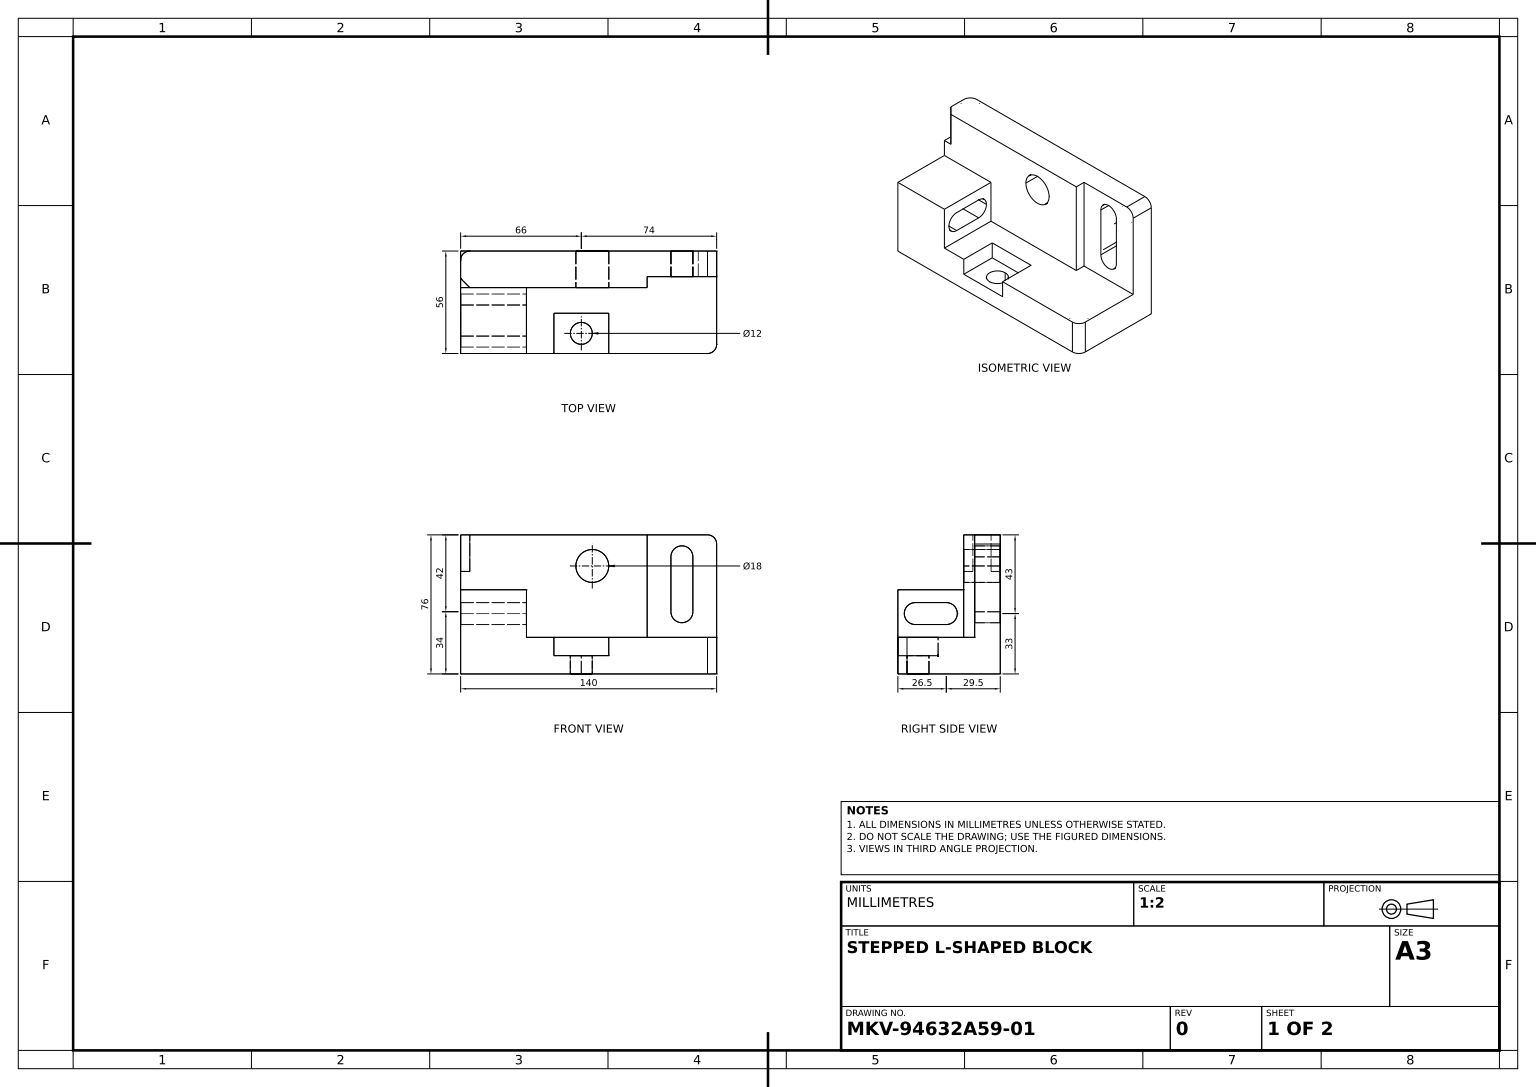
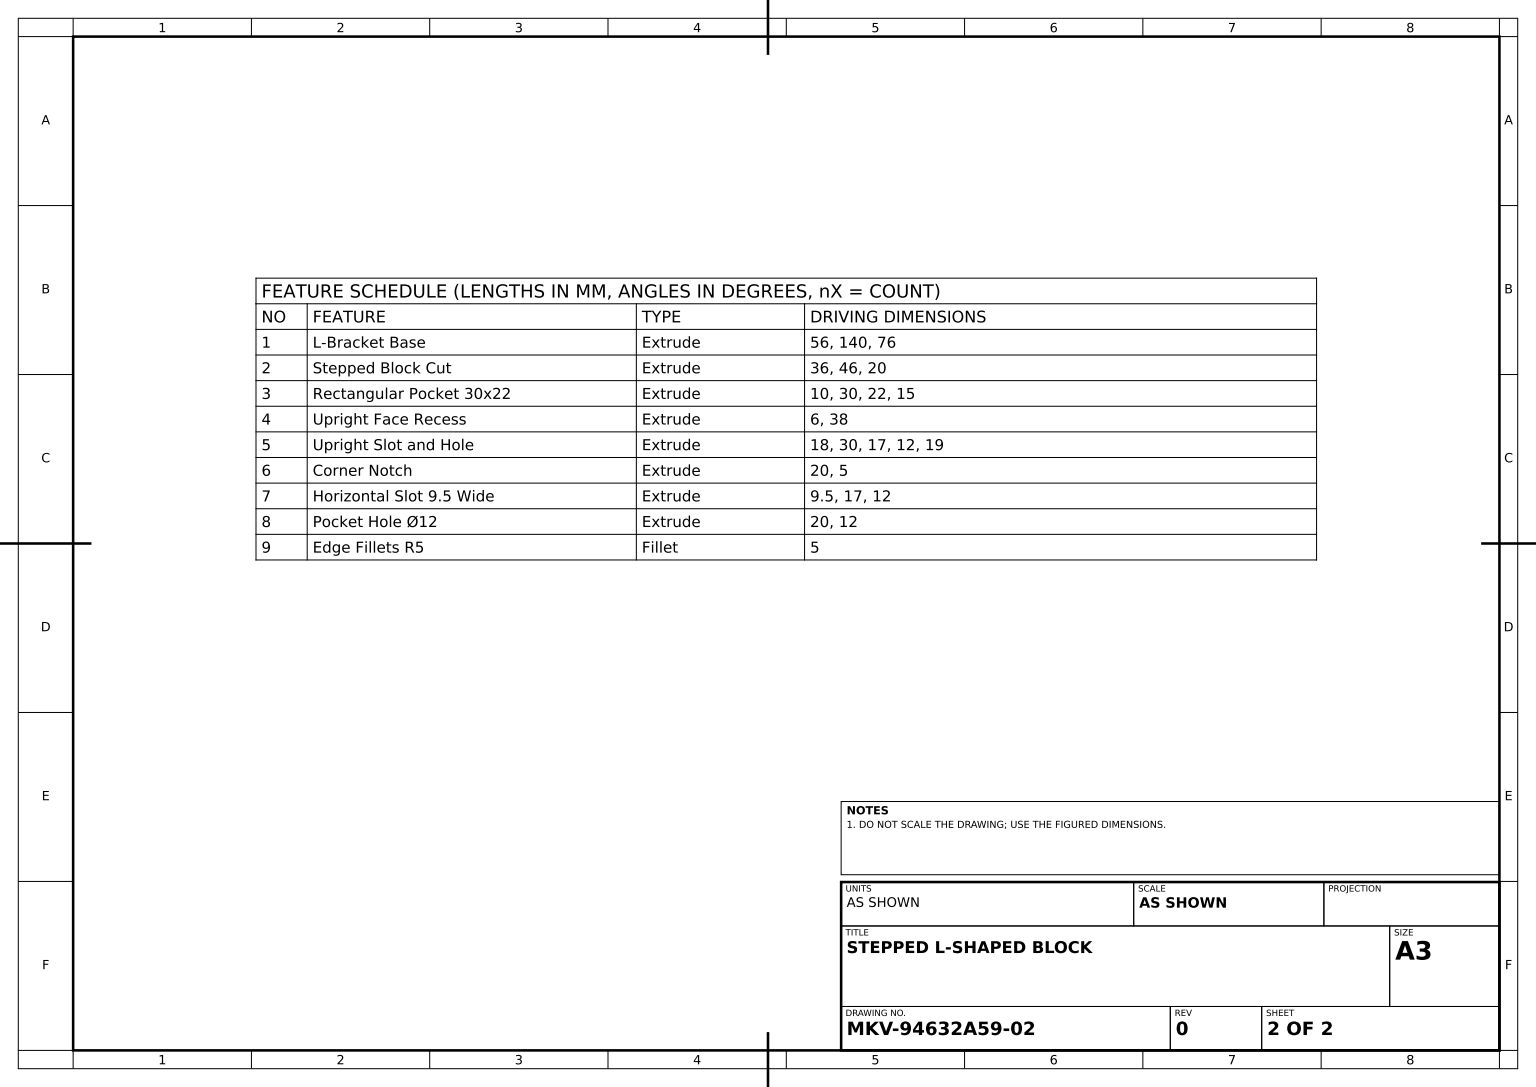
from build123d import *

# Parameters (mm, degrees)
L_BRACKET_PROFILE_SKETCH_W     = 140
L_BRACKET_PROFILE_SKETCH_H     = 76
L_BRACKET_BASE_DEPTH           = 28
STEPPED_BLOCK_CUT_DEPTH        = 36
RECTANGULAR_POCKET_SKETCH_W    = 30
RECTANGULAR_POCKET_SKETCH_H    = 22
RECTANGULAR_POCKET_30X22_DEPTH = 10
UPRIGHT_RECESS_SKETCH_W        = 38
UPRIGHT_RECESS_SKETCH_H        = 56
UPRIGHT_FACE_RECESS_DEPTH      = 6
UPRIGHT_SLOT_AND_HOLE_SKETCH_R = 9
UPRIGHT_SLOT_AND_HOLE_DEPTH    = 88.407093534
CORNER_NOTCH_DEPTH             = 20
HORIZONTAL_SLOT_9_5_WIDE_DEPTH = 115.210332282
POCKET_HOLE_SKETCH_R           = 6
POCKET_HOLE_12_DEPTH           = 20
EDGE_FILLETS_R5_R              = 5


with BuildPart() as part:
    # L-Bracket Profile Sketch → L-Bracket Base (new, symmetric)
    with BuildSketch(Plane.XY):
        Rectangle(L_BRACKET_PROFILE_SKETCH_W, L_BRACKET_PROFILE_SKETCH_H)
    extrude(amount=L_BRACKET_BASE_DEPTH, both=True)

    # Step Cut Sketch → Stepped Block Cut (cut)
    with BuildSketch(Plane.XY.offset(28)):
        Polygon((-70, 8), (-34, 8), (-34, -18), (70, -18), (70, 38), (-70, 38), align=None)
    extrude(amount=-STEPPED_BLOCK_CUT_DEPTH, mode=Mode.SUBTRACT)

    # Rectangular Pocket Sketch → Rectangular Pocket 30x22 (cut)
    with BuildSketch(Plane(origin=(0, -18, 0), x_dir=(1, 0, 0), z_dir=(0, 1, 0))):
        with Locations((-4, -17)):
            Rectangle(RECTANGULAR_POCKET_SKETCH_W, RECTANGULAR_POCKET_SKETCH_H)
    extrude(amount=-RECTANGULAR_POCKET_30X22_DEPTH, mode=Mode.SUBTRACT)

    # Upright Recess Sketch → Upright Face Recess (cut)
    with BuildSketch(Plane.XY.offset(-8)):
        with Locations((51, 10)):
            Rectangle(UPRIGHT_RECESS_SKETCH_W, UPRIGHT_RECESS_SKETCH_H)
    extrude(amount=-UPRIGHT_FACE_RECESS_DEPTH, mode=Mode.SUBTRACT)

    # Upright Slot and Hole Sketch → Upright Slot and Hole (cut, through all)
    with BuildSketch(Plane.XY.offset(-8)):
        with Locations((2, 21)):
            Circle(UPRIGHT_SLOT_AND_HOLE_SKETCH_R)
        with BuildLine():
            Line((45, -4), (45, 26))
            ThreePointArc((45, 26), (51, 32), (57, 26))
            Line((57, 26), (57, -4))
            ThreePointArc((57, -4), (51, -10), (45, -4))
        make_face()
    extrude(amount=-UPRIGHT_SLOT_AND_HOLE_DEPTH, mode=Mode.SUBTRACT)

    # Corner Notch Sketch → Corner Notch (cut)
    with BuildSketch(Plane(origin=(0, 38, 0), x_dir=(1, 0, 0), z_dir=(0, 1, 0))):
        Polygon((-70, 13), (-65, 8), (-70, 8), align=None)
        with BuildLine():
            Line((-70, 23), (-70, 28))
            Line((-70, 28), (-65, 28))
            ThreePointArc((-65, 28), (-68.535533906, 26.535533906), (-70, 23))
        make_face()
    extrude(amount=-CORNER_NOTCH_DEPTH, mode=Mode.SUBTRACT)

    # Horizontal Slot Sketch → Horizontal Slot 9.5 Wide (cut, through all)
    with BuildSketch(Plane(origin=(-34, 0, 0), x_dir=(0, 0, -1), z_dir=(1, 0, 0))):
        with BuildLine():
            Line((-18.5, 1), (-1.5, 1))
            ThreePointArc((-1.5, 1), (4.5, -5), (-1.5, -11))
            Line((-1.5, -11), (-18.5, -11))
            ThreePointArc((-18.5, -11), (-24.5, -5), (-18.5, 1))
        make_face()
    extrude(amount=-HORIZONTAL_SLOT_9_5_WIDE_DEPTH, mode=Mode.SUBTRACT)

    # Pocket Hole Sketch → Pocket Hole Ø12 (cut)
    with BuildSketch(Plane(origin=(0, -28, 0), x_dir=(1, 0, 0), z_dir=(0, 1, 0))):
        with Locations(Location((-4, -17, 0), (0, 0, 270))):
            Circle(POCKET_HOLE_SKETCH_R)
    extrude(amount=-POCKET_HOLE_12_DEPTH, mode=Mode.SUBTRACT)

    # Edge Fillets R5
    edge_fillets_r5_edges = [part.edges().sort_by_distance(p)[0] for p in [
        (70, -28, 28),
        (70, 38, -21),
    ]]
    fillet(edge_fillets_r5_edges, radius=EDGE_FILLETS_R5_R)


solid = part.part
